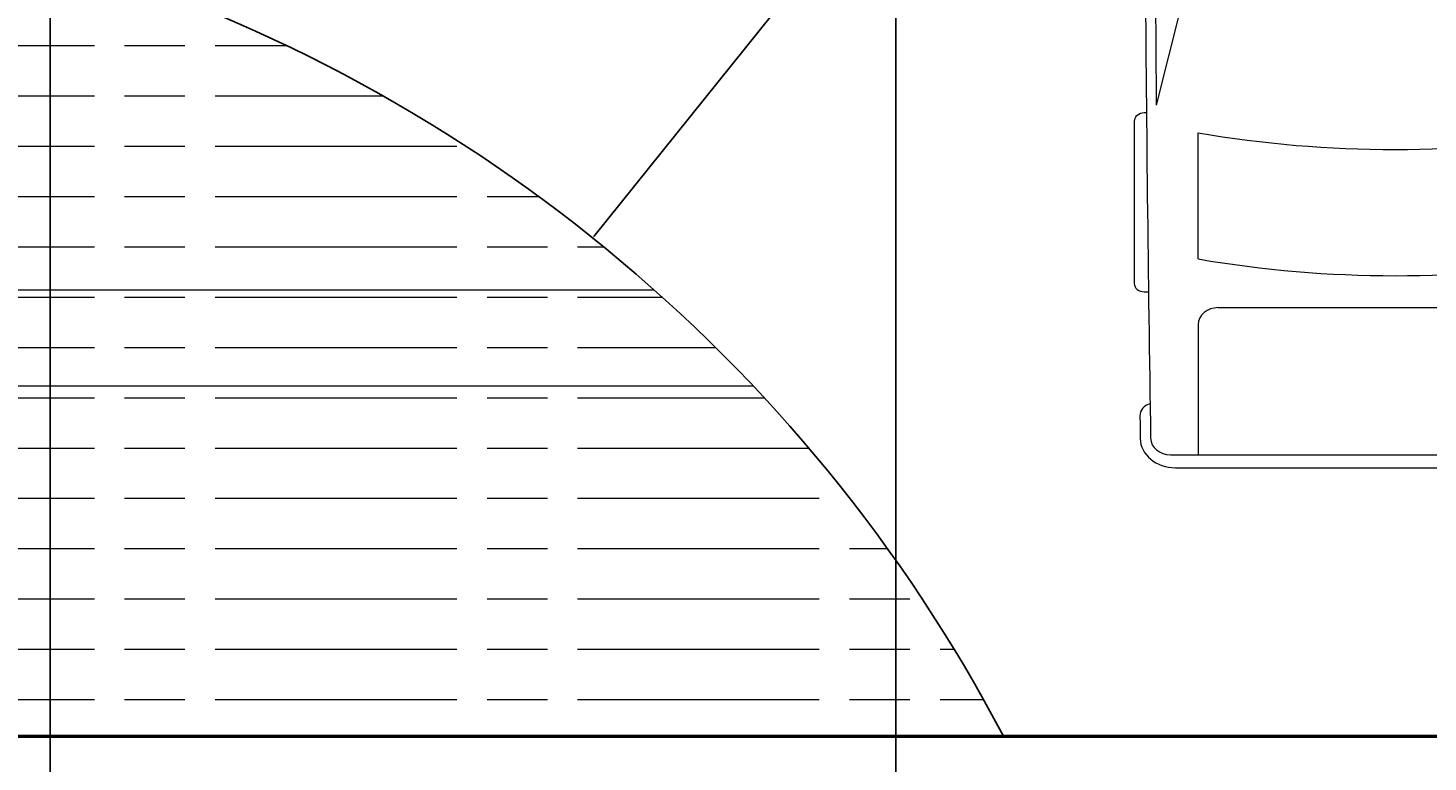
# Model space of a CAD drawing. Units: inches. Extents: x 5375 to 6084, y 16106 to 17259.
# Tile 6 of 32: x 5705 to 5844, y 16219 to 16292. Entities that reach past the tile are written whole.
import ezdxf

# ---------------------------------------------------------------- set-up
doc = ezdxf.new("R2010")
doc.units = ezdxf.units.IN
for name, color, linetype, lineweight in [('A-ANNO-DIMS', 2, 'Continuous', 18), ('C-PKNG-VEHI', 7, 'Continuous', 13), ('C-PVMT', 7, 'Continuous', 25), ('C-PVMT-PATT', 2, 'Continuous', 13), ('WALL', 6, 'Continuous', 50)]:
    doc.layers.add(name, color=color, linetype=linetype, lineweight=lineweight)
doc.styles.get("Standard").update_dxf_attribs({"font": 'arial.ttf'})
doc.dimstyles.get("Standard").update_dxf_attribs({"dimtxt": 0.18, "dimasz": 0.18, "dimexe": 0.18, "dimexo": 0.0625, "dimgap": 0.09, "dimtad": 0, "dimtih": 1, "dimtoh": 1, "dimdec": 4, "dimzin": 0, "dimdsep": 46, "dimtxsty": 'Standard', "dimcen": 0.09, "dimadec": 0, "dimazin": 0, "dimtfac": 1, "dimtdec": 4, "dimtofl": 0, "dimtmove": 0, "dimatfit": 3, "dimfxl": 1, "dimtolj": 1, "dimtzin": 0, "dimarcsym": 0})

# ---------------------------------------------------------------- blocks, each defined once
blk = doc.blocks.new('*U9')
for p, q in [((186.47, -33.5), (186.47, 33.5)), ((188.4, -32.76), (188.4, 32.76)), ((164.52, 26.39), (164.52, -26.39)), ((186.47, -10.53), (186.47, 10.53)), ((157.25, -29.35), (138.42, -29.35)), ((167.01, -29.35), (186.47, -29.35)), ((134.31, -35.6), (119.29, -31.78)), ((135.45, -37.07), (135.45, -37.41)), ((162.15, -37.41), (162.15, -36.77)), ((136.7, -38.89), (160.9, -38.89))]:
    blk.add_line(p, q)
for centre, major_axis, start_param, end_param in [((17.08, 0), (0, 147.02), 4.511394, 4.913384), ((35.91, 0), (0, 147.02), 4.511394, 4.913384), ((167.01, -26.39), (0, -2.96), 4.712389, 6.283185), ((183.98, -32.76), (0, -5.25), 0.013397, 1.570796), ((183.98, -33.5), (0, 2.96), 3.15499, 4.712389), ((64.48, 10555.62), (0, 10593.03), 3.138796, 3.15499), ((64.48, 10555.62), (0, -10591.55), 0.001152, 0.007828), ((136.7, -37.41), (0, -1.48), -1.570796, 0), ((160.9, -37.41), (0, 1.48), 3.141593, 4.712389), ((180.63, -35.84), (0, -2.22), -1.249894, 0.013017), ((64.48, 10556.36), (0, 10595.31), 3.15461, 3.15499)]:
    blk.add_ellipse(centre, major_axis=major_axis, ratio=0.842304, start_param=start_param, end_param=end_param)
blk = doc.blocks.new('*D38')
at = {"layer": 'A-ANNO-DIMS', "color": 0, "lineweight": -2, "transparency": 16777216}
for p, q in [((5791.62, 16513.52), (5791.62, 16106.48)), ((5707.62, 16507.52), (5707.62, 16106.48)), ((5707.8, 16106.66), (5749.4, 16106.66)), ((5791.44, 16106.66), (5749.84, 16106.66))]:
    blk.add_line(p, q, dxfattribs=at)
at = {"layer": 'A-ANNO-DIMS', "color": 0, "transparency": 16777216}
for points in [[(5707.8, 16106.69), (5707.8, 16106.63), (5707.62, 16106.66)], [(5791.44, 16106.69), (5791.44, 16106.63), (5791.62, 16106.66)]]:
    blk.add_solid(points, dxfattribs=at)
at = {"layer": 'Defpoints', "color": 0, "transparency": 16777216}
for p in [(5791.62, 16513.58), (5707.62, 16507.58), (5791.62, 16106.66)]:
    blk.add_point(p, dxfattribs=at)
at = {"layer": 'A-ANNO-DIMS', "color": 0, "transparency": 16777216, "insert": (5749.62, 16106.66), "char_height": 0.18, "attachment_point": 5}
blk.add_mtext('\\A1;84', dxfattribs=at)
blk = doc.blocks.new('*D51')
at = {"layer": 'A-ANNO-DIMS', "color": 0, "lineweight": -2, "transparency": 16777216}
for p, q in [((5820.47, 16344.39), (5761.62, 16271.02)), ((5820.65, 16344.39), (5820.47, 16344.39)), ((5663.14, 16148.34), (5663.32, 16148.34)), ((5663.23, 16148.25), (5663.23, 16148.43))]:
    blk.add_line(p, q, dxfattribs=at)
at = {"layer": 'A-ANNO-DIMS', "color": 0, "transparency": 16777216}
blk.add_solid([(5761.59, 16271.03), (5761.64, 16271), (5761.5, 16270.88)], dxfattribs=at)
at = {"layer": 'Defpoints', "color": 0, "transparency": 16777216}
for p in [(5761.5, 16270.88), (5663.23, 16148.34)]:
    blk.add_point(p, dxfattribs=at)
at = {"layer": 'A-ANNO-DIMS', "color": 0, "transparency": 16777216, "insert": (5821.2, 16344.39), "char_height": 0.18, "attachment_point": 5}
blk.add_mtext('\\A1;R157.07', dxfattribs=at)

msp = doc.modelspace()

# ---------------------------------------------------------------- hatches: boundary and pattern name
at = {"layer": 'C-PVMT-PATT'}
h = msp.add_hatch(dxfattribs=at)
h.set_pattern_fill('AR-B816C', color=256)
h.paths.add_polyline_path([(5707.6199, 16360.5793), (5479.6199, 16360.5793), (5479.6199, 16221.3785), (5802.2897, 16221.3785, 0.20288708), (5707.6199, 16299.0135)])
h = msp.add_hatch(dxfattribs=at)
h.set_pattern_fill('ACAD_ISO08W100', color=256)
h.paths.add_polyline_path([(5707.6199, 16360.5793), (5479.6199, 16360.5793), (5479.6199, 16221.3785), (5802.2897, 16221.3785, 0.20288708), (5707.6199, 16299.0135)])

# ---------------------------------------------------------------- linework, layer by layer
at = {"layer": 'C-PVMT'}
msp.add_arc((5663.2298, 16148.3446), 157.072, 27.708351, 73.583948, dxfattribs=at)
at = {"layer": 'WALL'}
msp.add_line((5479.6199, 16221.3785), (6022.6199, 16221.3785), dxfattribs=at)

# ---------------------------------------------------------------- block references
at = {"layer": 'C-PKNG-VEHI', "xscale": 0.6659567702331713, "yscale": 0.6659567702331713, "zscale": 0.6659567702331713, "rotation": 270}
msp.add_blockref('*U9', (5841.1969, 16373.5119), dxfattribs=at)

# ---------------------------------------------------------------- dimensions: what is measured, and where the dimension line sits
at = {"layer": 'A-ANNO-DIMS'}
dim = msp.add_linear_dim(base=(5791.6199, 16106.6631), p1=(5707.6199, 16507.5793), p2=(5791.6199, 16513.5793), dimstyle='Standard', override={"dimdec": 0, "dimlfac": 1, "dimrnd": 0, "dimzin": 0, "dimdsep": 46, "dimlunit": 2}, dxfattribs=at)
dim.commit()
dim.dimension.update_dxf_attribs({"geometry": '*D38', "text_midpoint": (5749.6199, 16106.6631)})
dim = msp.add_radius_dim(center=(5663.2298, 16148.3446), mpoint=(5761.504, 16270.8753), dimstyle='Standard', override={"dimdec": 2, "dimlfac": 1, "dimrnd": 0, "dimzin": 0, "dimdsep": 46, "dimlunit": 2}, dxfattribs=at)
dim.commit()
dim.dimension.update_dxf_attribs({"geometry": '*D51', "text_midpoint": (5821.1984, 16344.3937), "dimtype": 164})

doc.saveas('drawing.dxf')
